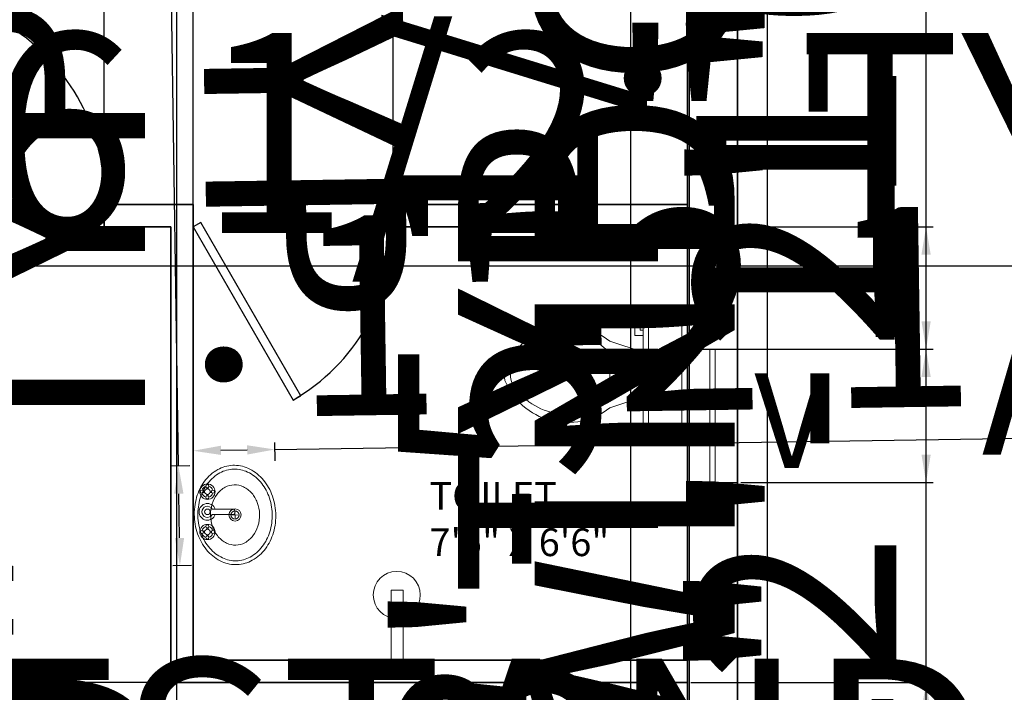
# Model space of a CAD drawing. Units: inches. Extents: x 2901 to 21549, y 2042 to 3828.
# Tile 6 of 10: x 3505 to 3682, y 3226 to 3347. Entities that reach past the tile are written whole.
import ezdxf

# ---------------------------------------------------------------- set-up
doc = ezdxf.new("R2010")
doc.units = ezdxf.units.IN
doc.layers.get('Defpoints').update_dxf_attribs({"color": 1})
for name, color, linetype, lineweight in [('A-ANNO-DIMS', 2, 'Continuous', 18), ('A-ANNO-TEXT', 7, 'Continuous', 18), ('A-AREA-IDEN', 7, 'Continuous', 18), ('A-DOOR', 3, 'Continuous', 25), ('A-FLOR-FIXT', 9, 'Continuous', 18), ('A-GLAZ', 4, 'Continuous', 18), ('A-WALL', 7, 'Continuous', 35)]:
    doc.layers.add(name, color=color, linetype=linetype, lineweight=lineweight)
doc.styles.get("Standard").update_dxf_attribs({"font": 'arial.ttf'})
doc.dimstyles.new('ISO-25', dxfattribs={"dimtxt": 36, "dimasz": 5, "dimexe": 1.25, "dimexo": 0.625, "dimtad": 1, "dimdec": 0, "dimlunit": 3, "dimtxsty": 'Standard', "dimcen": 2.5, "dimadec": 0, "dimazin": 0, "dimtfac": 1, "dimtdec": 0, "dimtmove": 0, "dimatfit": 3, "dimfxl": 1, "dimarcsym": 0})

# ---------------------------------------------------------------- blocks, each defined once
blk = doc.blocks.new('*U21')
for p, q in [((0, 0), (0, -6)), ((40, 0), (40, -6))]:
    blk.add_line(p, q)
blk.add_lwpolyline([(0, 0), (20, 34.64), (21.52, 33.77), (1.52, -0.88)], close=True)
blk.add_arc((0, 0), 40, 0, 60)
blk = doc.blocks.new('*U19')
for p, q in [((0, 0), (0, 6)), ((40, 0), (40, 6))]:
    blk.add_line(p, q)
blk.add_lwpolyline([(0, 0), (20, -34.64), (21.52, -33.77), (1.52, 0.88)], close=True)
blk.add_arc((0, 0), 40, 300, 0)
blk = doc.blocks.new('Toilet - top')
for p, q in [((9.5, -6), (9.5, -2)), ((-10, -8.5), (-8, -8.5)), ((-10, -9.5), (-10, -8.5)), ((-8, -8.5), (-8, -8)), ((-7, -8), (-7, -9.5)), ((-4, -8), (-6, -14)), ((4, -8), (6, -14)), ((-7, -9.5), (-10, -9.5)), ((4, -14), (-4, -14))]:
    blk.add_line(p, q)
blk.add_lwpolyline([(10.5, -8), (10.5, 0), (-10.5, 0), (-10.5, -8)], close=True)
for points in [[(8.5, -1), (-8.5, -1)], [(-9.5, -2), (-9.5, -6)], [(-8.5, -7), (8.5, -7)]]:
    blk.add_lwpolyline(points)
for centre, radius, start, end in [((-8.62, -1.88), 0.884, 81.8699, 188.1301), ((8.62, -1.88), 0.884, 351.8699, 98.1301), ((-8.62, -6.12), 0.884, 171.8699, 278.1301), ((8.62, -6.12), 0.884, 261.8699, 8.1301), ((3.52, -21.58), 12.17, 141.4691, 247.9714), ((4.2, -21.82), 11.33, 136.3677, 238.9468), ((-3.52, -21.58), 12.17, 292.0284, 38.5307), ((-4.2, -21.82), 11.33, 301.053, 43.6321), ((0, -27.88), 4, 245.7318, 294.2682), ((0, -29), 4, 254.8605, 285.1395)]:
    blk.add_arc(centre, radius, start, end)
blk = doc.blocks.new('Sink - Oval top')
for p, q in [((-1, 0), (1, 0)), ((0, 1), (0, -1))]:
    blk.add_line(p, q)
for points in [[(-12.23, 0.39, 0.117634), (-11.46, -3.36, 0.104469), (-8.88, -6.8, 0.090016), (-5.08, -9.07, 0.08192), (-0.32, -10.02, 0.08192), (4.49, -9.38, 0.090016), (8.42, -7.36, 0.104469), (11.22, -4.09, 0.117634), (12.23, -0.39, 0.117634), (11.46, 3.36, 0.104469), (8.88, 6.8, 0.090016), (5.08, 9.07, 0.08192), (0.32, 10.02, 0.08192), (-4.49, 9.38, 0.090016), (-8.42, 7.36, 0.104469), (-11.22, 4.09, 0.117634)], [(-11.29, 0.16, 0.118622), (-10.52, -3.25, 0.104678), (-8.07, -6.36, 0.089562), (-4.54, -8.37, 0.081185), (-0.13, -9.15, 0.081185), (4.3, -8.49, 0.089562), (7.89, -6.58, 0.104678), (10.42, -3.55, 0.118622), (11.29, -0.16, 0.118622), (10.52, 3.25, 0.104678), (8.07, 6.36, 0.089562), (4.54, 8.37, 0.081185), (0.13, 9.15, 0.081185), (-4.3, 8.49, 0.089562), (-7.89, 6.58, 0.104678), (-10.42, 3.55, 0.118622)], [(-7.42, 0.08, 0.118283), (-6.91, -2.17, 0.104607), (-5.29, -4.21, 0.089718), (-2.97, -5.53, 0.081436), (-0.07, -6.04, 0.081436), (2.84, -5.59, 0.089718), (5.2, -4.33, 0.104607), (6.86, -2.32, 0.118283), (7.42, -0.08, 0.118283), (6.91, 2.17, 0.104607), (5.29, 4.21, 0.089718), (2.97, 5.53, 0.081436), (0.07, 6.04, 0.081436), (-2.84, 5.59, 0.089718), (-5.2, 4.33, 0.104607), (-6.86, 2.32, 0.118283)]]:
    blk.add_lwpolyline(points, format="xyb", close=True)
for radius in [1.5, 1]:
    blk.add_circle((0, 0), radius)
blk = doc.blocks.new('Faucet - Bathroom top')
for p, q in [((-4.107, 0.125), (-4.375, 0.125)), ((-3.75, 0.4788), (-3.75, 0.75)), ((-3.5, 0.482), (-3.5, 0.75)), ((-3.1461, 0.125), (-2.875, 0.125)), ((3.143, 0.125), (2.875, 0.125)), ((3.5, 0.4788), (3.5, 0.75)), ((3.75, 0.482), (3.75, 0.75)), ((4.1039, 0.125), (4.375, 0.125)), ((-4.1039, -0.125), (-4.375, -0.125)), ((-3.75, -0.4821), (-3.75, -0.75)), ((-3.5, -0.4789), (-3.5, -0.75)), ((-3.143, -0.125), (-2.875, -0.125)), ((-0.5, -0.8639), (-0.5, -4.5)), ((0.5, -4.5), (0.5, -0.8631)), ((3.1461, -0.125), (2.875, -0.125)), ((3.5, -0.4821), (3.5, -0.75)), ((3.75, -0.4789), (3.75, -0.75)), ((4.107, -0.125), (4.375, -0.125))]:
    blk.add_line(p, q)
for centre, radius in [((-3.625, 0), 1.375), ((-4.625, 0), 0.2795), ((-3.625, 0), 0.5), ((-3.625, 1), 0.2795), ((-2.625, 0), 0.2795), ((0, 0), 0.5), ((3.625, 0), 1.375), ((2.625, 0), 0.2795), ((3.625, 0), 0.5), ((3.625, 1), 0.2795), ((4.625, 0), 0.2795), ((-3.625, -1), 0.2795), ((3.625, -1), 0.2795)]:
    blk.add_circle(centre, radius)
for centre, radius, start, end in [((-3.625, 0), 1, 105.2407, 164.2093), ((-3.625, 0), 1, 16.44125, 74.07887), ((0, 0), 1.5, 289.6514, 250.3603), ((0, 0), 1, 300.3431, 239.7554), ((3.625, 0), 1, 106.12, 164.0884), ((3.625, 0), 1, 16.23422, 73.90469), ((-3.625, 0), 1, 196.2342, 253.9047), ((-3.625, 0), 1, 286.12, 344.0884), ((3.625, 0), 1, 196.4413, 254.0789), ((3.625, 0), 1, 285.2407, 344.2093), ((0, -4.5), 0.5, 180, 0)]:
    blk.add_arc(centre, radius, start, end)
blk = doc.blocks.new('*D36')
at = {"layer": 'A-ANNO-DIMS', "color": 0, "lineweight": -2, "transparency": 16777216}
for p, q in [((3639.47, 3192.64), (3639.47, 3654.44)), ((3634.69, 3192.64), (3640.72, 3192.64)), ((3639.47, 3161.64), (3639.47, 3187.64)), ((3634.69, 3156.64), (3640.72, 3156.64))]:
    blk.add_line(p, q, dxfattribs=at)
at = {"layer": 'A-ANNO-DIMS', "color": 0, "transparency": 16777216}
for points in [[(3638.64, 3187.64), (3640.3, 3187.64), (3639.47, 3192.64)], [(3638.64, 3161.64), (3640.3, 3161.64), (3639.47, 3156.64)]]:
    blk.add_solid(points, dxfattribs=at)
at = {"layer": 'Defpoints', "color": 0, "transparency": 16777216}
for p in [(3634.07, 3192.64), (3639.47, 3192.64), (3634.07, 3156.64)]:
    blk.add_point(p, dxfattribs=at)
at = {"layer": 'A-ANNO-DIMS', "color": 0, "transparency": 16777216, "insert": (3620.21, 3426.04), "char_height": 36, "attachment_point": 5, "rotation": 90}
blk.add_mtext('WINDOW 3\'-0" TYP.', dxfattribs=at)
blk = doc.blocks.new('*D38')
at = {"layer": 'A-ANNO-DIMS', "color": 0, "lineweight": -2, "transparency": 16777216}
for p, q in [((3343.07, 3191.34), (3343.07, 3188.58)), ((3357.29, 3191.34), (3357.29, 3188.58)), ((3348.07, 3189.83), (3352.29, 3189.83)), ((3357.29, 3189.83), (3922.11, 3189.83))]:
    blk.add_line(p, q, dxfattribs=at)
at = {"layer": 'A-ANNO-DIMS', "color": 0, "transparency": 16777216}
for points in [[(3348.07, 3190.67), (3348.07, 3189), (3343.07, 3189.83)], [(3352.29, 3190.67), (3352.29, 3189), (3357.29, 3189.83)]]:
    blk.add_solid(points, dxfattribs=at)
at = {"layer": 'Defpoints', "color": 0, "transparency": 16777216}
for p in [(3343.07, 3191.97), (3357.29, 3191.97), (3357.29, 3189.83)]:
    blk.add_point(p, dxfattribs=at)
at = {"layer": 'A-ANNO-DIMS', "color": 0, "transparency": 16777216, "insert": (3642.2, 3209.07), "char_height": 36, "attachment_point": 5}
blk.add_mtext('NIGHTSTAND 1\'-2" TYP.', dxfattribs=at)
blk = doc.blocks.new('*D42')
at = {"layer": 'A-ANNO-DIMS', "color": 0, "lineweight": -2, "transparency": 16777216}
for p, q in [((3533.42, 3266.44), (3528.38, 3599.53)), ((3535.49, 3266.47), (3532.17, 3266.42)), ((3533.62, 3253.49), (3533.5, 3261.44)), ((3535.76, 3248.52), (3532.44, 3248.47))]:
    blk.add_line(p, q, dxfattribs=at)
at = {"layer": 'A-ANNO-DIMS', "color": 0, "transparency": 16777216}
for points in [[(3534.33, 3261.45), (3532.66, 3261.43), (3533.42, 3266.44)], [(3534.45, 3253.5), (3532.78, 3253.48), (3533.69, 3248.49)]]:
    blk.add_solid(points, dxfattribs=at)
at = {"layer": 'Defpoints', "color": 0, "transparency": 16777216}
for p in [(3533.42, 3266.44), (3536.11, 3266.48), (3536.39, 3248.53)]:
    blk.add_point(p, dxfattribs=at)
at = {"layer": 'A-ANNO-DIMS', "color": 0, "transparency": 16777216, "insert": (3549.86, 3435.77), "char_height": 36, "attachment_point": 5, "rotation": 270.8679}
blk.add_mtext('LAV 1\'-6" TYP.', dxfattribs=at)
blk = doc.blocks.new('*D43')
at = {"layer": 'A-ANNO-DIMS', "color": 0, "lineweight": -2, "transparency": 16777216}
for p, q in [((3550.8, 3269.4), (3856.95, 3274.04)), ((3536.1, 3267.11), (3536.05, 3270.42)), ((3550.83, 3267.33), (3550.78, 3270.65)), ((3541.07, 3269.25), (3545.8, 3269.32))]:
    blk.add_line(p, q, dxfattribs=at)
at = {"layer": 'A-ANNO-DIMS', "color": 0, "transparency": 16777216}
for points in [[(3541.06, 3270.08), (3541.09, 3268.42), (3536.07, 3269.17)], [(3545.78, 3270.16), (3545.81, 3268.49), (3550.8, 3269.4)]]:
    blk.add_solid(points, dxfattribs=at)
at = {"layer": 'Defpoints', "color": 0, "transparency": 16777216}
for p in [(3550.8, 3269.4), (3536.11, 3266.48), (3550.84, 3266.71)]:
    blk.add_point(p, dxfattribs=at)
at = {"layer": 'A-ANNO-DIMS', "color": 0, "transparency": 16777216, "insert": (3706.08, 3290.99), "char_height": 36, "attachment_point": 5, "rotation": 0.8679}
blk.add_mtext('1\'-2 1/2" TYP.', dxfattribs=at)
blk = doc.blocks.new('*D45')
at = {"layer": 'A-ANNO-DIMS', "color": 0, "lineweight": -2, "transparency": 16777216}
for p, q in [((3419.19, 3302.47), (3414.19, 3302.47)), ((3424.19, 3301.6), (3424.19, 3303.72)), ((3424.19, 3302.47), (3430.69, 3302.47)), ((3430.69, 3301.6), (3430.69, 3303.72)), ((3435.69, 3302.47), (3745.26, 3302.47))]:
    blk.add_line(p, q, dxfattribs=at)
at = {"layer": 'A-ANNO-DIMS', "color": 0, "transparency": 16777216}
for points in [[(3419.19, 3303.31), (3419.19, 3301.64), (3424.19, 3302.47)], [(3435.69, 3303.31), (3435.69, 3301.64), (3430.69, 3302.47)]]:
    blk.add_solid(points, dxfattribs=at)
at = {"layer": 'Defpoints', "color": 0, "transparency": 16777216}
for p in [(3430.69, 3302.47), (3424.19, 3300.97), (3430.69, 3300.97)]:
    blk.add_point(p, dxfattribs=at)
at = {"layer": 'A-ANNO-DIMS', "color": 0, "transparency": 16777216, "insert": (3592.98, 3321.71), "char_height": 36, "attachment_point": 5}
blk.add_mtext('0\'-6 1/2" TYP.', dxfattribs=at)
blk = doc.blocks.new('*D46')
at = {"layer": 'A-ANNO-DIMS', "color": 0, "lineweight": -2, "transparency": 16777216}
for p, q in [((3545.07, 3370.05), (3545.07, 3357.42)), ((3625.07, 3370.05), (3625.07, 3357.42)), ((3550.07, 3358.67), (3620.07, 3358.67)), ((3625.07, 3358.67), (4160.88, 3358.67))]:
    blk.add_line(p, q, dxfattribs=at)
at = {"layer": 'A-ANNO-DIMS', "color": 0, "transparency": 16777216}
for points in [[(3550.07, 3359.51), (3550.07, 3357.84), (3545.07, 3358.67)], [(3620.07, 3359.51), (3620.07, 3357.84), (3625.07, 3358.67)]]:
    blk.add_solid(points, dxfattribs=at)
at = {"layer": 'Defpoints', "color": 0, "transparency": 16777216}
for p in [(3545.07, 3370.67), (3625.07, 3370.67), (3625.07, 3358.67)]:
    blk.add_point(p, dxfattribs=at)
at = {"layer": 'A-ANNO-DIMS', "color": 0, "transparency": 16777216, "insert": (3895.48, 3379.02), "char_height": 36, "attachment_point": 5}
blk.add_mtext('QUEEN BED 6\'-8" TYP.', dxfattribs=at)
blk = doc.blocks.new('*D47')
at = {"layer": 'A-ANNO-DIMS', "color": 0, "lineweight": -2, "transparency": 16777216}
for p, q in [((3544.44, 3430.67), (3531.82, 3430.67)), ((3533.07, 3425.67), (3533.07, 3375.67)), ((3544.44, 3370.67), (3531.82, 3370.67)), ((3533.07, 3370.67), (3533.07, 3144.99))]:
    blk.add_line(p, q, dxfattribs=at)
at = {"layer": 'A-ANNO-DIMS', "color": 0, "transparency": 16777216}
for points in [[(3532.24, 3425.67), (3533.9, 3425.67), (3533.07, 3430.67)], [(3532.24, 3375.67), (3533.9, 3375.67), (3533.07, 3370.67)]]:
    blk.add_solid(points, dxfattribs=at)
at = {"layer": 'Defpoints', "color": 0, "transparency": 16777216}
for p in [(3545.07, 3430.67), (3533.07, 3370.67), (3545.07, 3370.67)]:
    blk.add_point(p, dxfattribs=at)
at = {"layer": 'A-ANNO-DIMS', "color": 0, "transparency": 16777216, "insert": (3514.06, 3255.33), "char_height": 36, "attachment_point": 5, "rotation": 90}
blk.add_mtext('5\'-0" TYP.', dxfattribs=at)
blk = doc.blocks.new('*D50')
at = {"layer": 'A-ANNO-DIMS', "color": 0, "lineweight": -2, "transparency": 16777216}
for p, q in [((3599.61, 3100.68), (3599.61, 3096.69)), ((3622.08, 3100.68), (3622.08, 3096.69)), ((3604.61, 3097.94), (3617.08, 3097.94)), ((3622.08, 3097.94), (4251.18, 3097.94))]:
    blk.add_line(p, q, dxfattribs=at)
at = {"layer": 'A-ANNO-DIMS', "color": 0, "transparency": 16777216}
for points in [[(3604.61, 3098.77), (3604.61, 3097.1), (3599.61, 3097.94)], [(3617.08, 3098.77), (3617.08, 3097.1), (3622.08, 3097.94)]]:
    blk.add_solid(points, dxfattribs=at)
at = {"layer": 'Defpoints', "color": 0, "transparency": 16777216}
for p in [(3599.61, 3101.31), (3622.08, 3101.31), (3622.08, 3097.94)]:
    blk.add_point(p, dxfattribs=at)
at = {"layer": 'A-ANNO-DIMS', "color": 0, "transparency": 16777216, "insert": (3939.13, 3117.18), "char_height": 36, "attachment_point": 5}
blk.add_mtext('END TABLE 1\'-10 1/2" TYP.', dxfattribs=at)
blk = doc.blocks.new('*D51')
at = {"layer": 'A-ANNO-DIMS', "color": 0, "lineweight": -2, "transparency": 16777216}
for p, q in [((3625.45, 3119.55), (3625.45, 3341.85)), ((3622.7, 3119.55), (3626.7, 3119.55)), ((3625.45, 3106.31), (3625.45, 3114.55)), ((3622.7, 3101.31), (3626.7, 3101.31))]:
    blk.add_line(p, q, dxfattribs=at)
at = {"layer": 'A-ANNO-DIMS', "color": 0, "transparency": 16777216}
for points in [[(3624.61, 3114.55), (3626.28, 3114.55), (3625.45, 3119.55)], [(3624.61, 3106.31), (3626.28, 3106.31), (3625.45, 3101.31)]]:
    blk.add_solid(points, dxfattribs=at)
at = {"layer": 'Defpoints', "color": 0, "transparency": 16777216}
for p in [(3622.08, 3119.55), (3625.45, 3119.55), (3622.08, 3101.31)]:
    blk.add_point(p, dxfattribs=at)
at = {"layer": 'A-ANNO-DIMS', "color": 0, "transparency": 16777216, "insert": (3606.44, 3233.2), "char_height": 36, "attachment_point": 5, "rotation": 90}
blk.add_mtext('1\'-6" TYP.', dxfattribs=at)
blk = doc.blocks.new('*D54')
at = {"layer": 'A-ANNO-DIMS', "color": 0, "lineweight": -2, "transparency": 16777216}
for p, q in [((3536.12, 3164.87), (3536.12, 3153.97)), ((3604.61, 3164.87), (3604.61, 3153.97)), ((3541.12, 3155.22), (3599.61, 3155.22)), ((3604.61, 3155.22), (4090.43, 3155.22))]:
    blk.add_line(p, q, dxfattribs=at)
at = {"layer": 'A-ANNO-DIMS', "color": 0, "transparency": 16777216}
for points in [[(3541.12, 3156.05), (3541.12, 3154.38), (3536.12, 3155.22)], [(3599.61, 3156.05), (3599.61, 3154.38), (3604.61, 3155.22)]]:
    blk.add_solid(points, dxfattribs=at)
at = {"layer": 'Defpoints', "color": 0, "transparency": 16777216}
for p in [(3536.12, 3165.49), (3604.61, 3165.49), (3604.61, 3155.22)]:
    blk.add_point(p, dxfattribs=at)
at = {"layer": 'A-ANNO-DIMS', "color": 0, "transparency": 16777216, "insert": (3850.02, 3174.46), "char_height": 36, "attachment_point": 5}
blk.add_mtext('DINING SET 5\'-8 1/2"', dxfattribs=at)
blk = doc.blocks.new('*D55')
at = {"layer": 'A-ANNO-DIMS', "color": 0, "lineweight": -2, "transparency": 16777216}
for p, q in [((3614.88, 3206.89), (3614.88, 3392.69)), ((3605.24, 3206.89), (3616.13, 3206.89)), ((3614.88, 3170.49), (3614.88, 3201.89)), ((3605.24, 3165.49), (3616.13, 3165.49))]:
    blk.add_line(p, q, dxfattribs=at)
at = {"layer": 'A-ANNO-DIMS', "color": 0, "transparency": 16777216}
for points in [[(3614.05, 3201.89), (3615.72, 3201.89), (3614.88, 3206.89)], [(3614.05, 3170.49), (3615.72, 3170.49), (3614.88, 3165.49)]]:
    blk.add_solid(points, dxfattribs=at)
at = {"layer": 'Defpoints', "color": 0, "transparency": 16777216}
for p in [(3604.61, 3206.89), (3614.88, 3206.89), (3604.61, 3165.49)]:
    blk.add_point(p, dxfattribs=at)
at = {"layer": 'A-ANNO-DIMS', "color": 0, "transparency": 16777216, "insert": (3595.63, 3302.29), "char_height": 36, "attachment_point": 5, "rotation": 90}
blk.add_mtext('3\'-5 1/2"', dxfattribs=at)
blk = doc.blocks.new('*D67')
at = {"layer": 'A-ANNO-DIMS', "color": 0, "lineweight": -2, "transparency": 16777216}
for p, q in [((3484.07, 3013.1), (3484.07, 3509.68)), ((3489.07, 3508.43), (3620.07, 3508.43)), ((3625.07, 3228.1), (3625.07, 3509.68))]:
    blk.add_line(p, q, dxfattribs=at)
at = {"layer": 'A-ANNO-DIMS', "color": 0, "transparency": 16777216}
for points in [[(3489.07, 3509.26), (3489.07, 3507.59), (3484.07, 3508.43)], [(3620.07, 3509.26), (3620.07, 3507.59), (3625.07, 3508.43)]]:
    blk.add_solid(points, dxfattribs=at)
at = {"layer": 'Defpoints', "color": 0, "transparency": 16777216}
for p in [(3625.07, 3508.43), (3625.07, 3227.48), (3484.07, 3012.48)]:
    blk.add_point(p, dxfattribs=at)
at = {"layer": 'A-ANNO-DIMS', "color": 0, "transparency": 16777216, "insert": (3554.57, 3527.43), "char_height": 36, "attachment_point": 5}
blk.add_mtext('11\'-9"', dxfattribs=at)
blk = doc.blocks.new('*D68')
at = {"layer": 'A-ANNO-DIMS', "color": 0, "lineweight": -2, "transparency": 16777216}
for p, q in [((3531.44, 3227.48), (3298.87, 3227.48)), ((3300.12, 3017.48), (3300.12, 3222.48)), ((3483.44, 3012.48), (3298.87, 3012.48))]:
    blk.add_line(p, q, dxfattribs=at)
at = {"layer": 'A-ANNO-DIMS', "color": 0, "transparency": 16777216}
for points in [[(3299.29, 3222.48), (3300.95, 3222.48), (3300.12, 3227.48)], [(3299.29, 3017.48), (3300.95, 3017.48), (3300.12, 3012.48)]]:
    blk.add_solid(points, dxfattribs=at)
at = {"layer": 'Defpoints', "color": 0, "transparency": 16777216}
for p in [(3300.12, 3227.48), (3532.07, 3227.48), (3484.07, 3012.48)]:
    blk.add_point(p, dxfattribs=at)
at = {"layer": 'A-ANNO-DIMS', "color": 0, "transparency": 16777216, "insert": (3281.42, 3119.98), "char_height": 36, "attachment_point": 5, "rotation": 90}
blk.add_mtext('17\'-11"', dxfattribs=at)
blk = doc.blocks.new('*D69')
at = {"layer": 'A-ANNO-DIMS', "color": 0, "lineweight": -2, "transparency": 16777216}
for p, q in [((3668.02, 3287.47), (3668.02, 3390.03)), ((3634.69, 3287.47), (3669.27, 3287.47)), ((3668.02, 3268.47), (3668.02, 3282.47)), ((3634.69, 3263.47), (3669.27, 3263.47))]:
    blk.add_line(p, q, dxfattribs=at)
at = {"layer": 'A-ANNO-DIMS', "color": 0, "transparency": 16777216}
for points in [[(3667.19, 3282.47), (3668.85, 3282.47), (3668.02, 3287.47)], [(3667.19, 3268.47), (3668.85, 3268.47), (3668.02, 3263.47)]]:
    blk.add_solid(points, dxfattribs=at)
at = {"layer": 'Defpoints', "color": 0, "transparency": 16777216}
for p in [(3634.07, 3287.47), (3668.02, 3287.47), (3634.07, 3263.47)]:
    blk.add_point(p, dxfattribs=at)
at = {"layer": 'A-ANNO-DIMS', "color": 0, "transparency": 16777216, "insert": (3649.01, 3341.25), "char_height": 36, "attachment_point": 5, "rotation": 90}
blk.add_mtext('2\'-0"', dxfattribs=at)
blk = doc.blocks.new('*D70')
at = {"layer": 'A-ANNO-DIMS', "color": 0, "lineweight": -2, "transparency": 16777216}
for p, q in [((3668.02, 3309.48), (3668.02, 3436.01)), ((3625.69, 3309.48), (3669.27, 3309.48)), ((3668.02, 3292.47), (3668.02, 3304.48)), ((3625.69, 3287.47), (3669.27, 3287.47))]:
    blk.add_line(p, q, dxfattribs=at)
at = {"layer": 'A-ANNO-DIMS', "color": 0, "transparency": 16777216}
for points in [[(3667.19, 3304.48), (3668.85, 3304.48), (3668.02, 3309.48)], [(3667.19, 3292.47), (3668.85, 3292.47), (3668.02, 3287.47)]]:
    blk.add_solid(points, dxfattribs=at)
at = {"layer": 'Defpoints', "color": 0, "transparency": 16777216}
for p in [(3625.07, 3309.48), (3668.02, 3309.48), (3625.07, 3287.47)]:
    blk.add_point(p, dxfattribs=at)
at = {"layer": 'A-ANNO-DIMS', "color": 0, "transparency": 16777216, "insert": (3649.01, 3375.24), "char_height": 36, "attachment_point": 5, "rotation": 90}
blk.add_mtext('1\'-10"', dxfattribs=at)
blk = doc.blocks.new('*D71')
at = {"layer": 'A-ANNO-DIMS', "color": 0, "lineweight": -2, "transparency": 16777216}
for p, q in [((3536.07, 3310.1), (3536.07, 3509.68)), ((3541.07, 3508.43), (3567.07, 3508.43)), ((3572.07, 3310.1), (3572.07, 3509.68)), ((3572.07, 3508.43), (3673.99, 3508.43))]:
    blk.add_line(p, q, dxfattribs=at)
at = {"layer": 'A-ANNO-DIMS', "color": 0, "transparency": 16777216}
for points in [[(3541.07, 3509.26), (3541.07, 3507.59), (3536.07, 3508.43)], [(3567.07, 3509.26), (3567.07, 3507.59), (3572.07, 3508.43)]]:
    blk.add_solid(points, dxfattribs=at)
at = {"layer": 'Defpoints', "color": 0, "transparency": 16777216}
for p in [(3572.07, 3508.43), (3536.07, 3309.48), (3572.07, 3309.48)]:
    blk.add_point(p, dxfattribs=at)
at = {"layer": 'A-ANNO-DIMS', "color": 0, "transparency": 16777216, "insert": (3625.53, 3527.45), "char_height": 36, "attachment_point": 5}
blk.add_mtext('3\'-0"', dxfattribs=at)
blk = doc.blocks.new('*D73')
at = {"layer": 'A-ANNO-DIMS', "color": 0, "lineweight": -2, "transparency": 16777216}
for p, q in [((3668.02, 3058.19), (3668.02, 3244)), ((3625.69, 3058.19), (3669.27, 3058.19)), ((3668.02, 3017.48), (3668.02, 3053.19)), ((3625.69, 3012.48), (3669.27, 3012.48))]:
    blk.add_line(p, q, dxfattribs=at)
at = {"layer": 'A-ANNO-DIMS', "color": 0, "transparency": 16777216}
for points in [[(3667.19, 3053.19), (3668.85, 3053.19), (3668.02, 3058.19)], [(3667.19, 3017.48), (3668.85, 3017.48), (3668.02, 3012.48)]]:
    blk.add_solid(points, dxfattribs=at)
at = {"layer": 'Defpoints', "color": 0, "transparency": 16777216}
for p in [(3625.07, 3058.19), (3668.02, 3058.19), (3625.07, 3012.48)]:
    blk.add_point(p, dxfattribs=at)
at = {"layer": 'A-ANNO-DIMS', "color": 0, "transparency": 16777216, "insert": (3648.77, 3153.6), "char_height": 36, "attachment_point": 5, "rotation": 90}
blk.add_mtext('3\'-9 1/2"', dxfattribs=at)
blk = doc.blocks.new('*D74')
at = {"layer": 'A-ANNO-DIMS', "color": 0, "lineweight": -2, "transparency": 16777216}
for p, q in [((3668.02, 3227.48), (3668.02, 3358.01)), ((3625.69, 3227.48), (3669.27, 3227.48)), ((3668.02, 3197.64), (3668.02, 3222.48)), ((3625.69, 3192.64), (3669.27, 3192.64))]:
    blk.add_line(p, q, dxfattribs=at)
at = {"layer": 'A-ANNO-DIMS', "color": 0, "transparency": 16777216}
for points in [[(3667.19, 3222.48), (3668.85, 3222.48), (3668.02, 3227.48)], [(3667.19, 3197.64), (3668.85, 3197.64), (3668.02, 3192.64)]]:
    blk.add_solid(points, dxfattribs=at)
at = {"layer": 'Defpoints', "color": 0, "transparency": 16777216}
for p in [(3625.07, 3227.48), (3668.02, 3227.48), (3625.07, 3192.64)]:
    blk.add_point(p, dxfattribs=at)
at = {"layer": 'A-ANNO-DIMS', "color": 0, "transparency": 16777216, "insert": (3649.32, 3295.24), "char_height": 36, "attachment_point": 5, "rotation": 90}
blk.add_mtext('2\'-11"', dxfattribs=at)
blk = doc.blocks.new('*D77')
at = {"layer": 'A-ANNO-DIMS', "color": 0, "lineweight": -2, "transparency": 16777216}
for p, q in [((3475.07, 3508.43), (3470.07, 3508.43)), ((3480.07, 3310.1), (3480.07, 3509.68)), ((3480.07, 3508.43), (3484.07, 3508.43)), ((3484.07, 3310.1), (3484.07, 3509.68)), ((3489.07, 3508.43), (3591.02, 3508.43))]:
    blk.add_line(p, q, dxfattribs=at)
at = {"layer": 'A-ANNO-DIMS', "color": 0, "transparency": 16777216}
for points in [[(3475.07, 3509.26), (3475.07, 3507.59), (3480.07, 3508.43)], [(3489.07, 3509.26), (3489.07, 3507.59), (3484.07, 3508.43)]]:
    blk.add_solid(points, dxfattribs=at)
at = {"layer": 'Defpoints', "color": 0, "transparency": 16777216}
for p in [(3484.07, 3508.43), (3480.07, 3309.48), (3484.07, 3309.48)]:
    blk.add_point(p, dxfattribs=at)
at = {"layer": 'A-ANNO-DIMS', "color": 0, "transparency": 16777216, "insert": (3542.54, 3527.43), "char_height": 36, "attachment_point": 5}
blk.add_mtext('0\'-4"', dxfattribs=at)
blk = doc.blocks.new('*D78')
at = {"layer": 'A-ANNO-DIMS', "color": 0, "lineweight": -2, "transparency": 16777216}
for p, q in [((3343.07, 3230.85), (3343.07, 2839.28)), ((3366.66, 3230.85), (3366.66, 2839.28)), ((3348.07, 2840.53), (3361.66, 2840.53)), ((3366.66, 2840.53), (3577.07, 2840.53))]:
    blk.add_line(p, q, dxfattribs=at)
at = {"layer": 'A-ANNO-DIMS', "color": 0, "transparency": 16777216}
for points in [[(3348.07, 2841.36), (3348.07, 2839.69), (3343.07, 2840.53)], [(3361.66, 2841.36), (3361.66, 2839.69), (3366.66, 2840.53)]]:
    blk.add_solid(points, dxfattribs=at)
at = {"layer": 'Defpoints', "color": 0, "transparency": 16777216}
for p in [(3343.07, 3231.48), (3366.66, 3231.48), (3366.66, 2840.53)]:
    blk.add_point(p, dxfattribs=at)
at = {"layer": 'A-ANNO-DIMS', "color": 0, "transparency": 16777216, "insert": (3474.37, 2859.77), "char_height": 36, "attachment_point": 5}
blk.add_mtext('1\'-11 1/2"', dxfattribs=at)
blk = doc.blocks.new('*D81')
at = {"layer": 'A-ANNO-DIMS', "color": 0, "lineweight": -2, "transparency": 16777216}
for p, q in [((3444.07, 3314.1), (3444.07, 3509.68)), ((3449.07, 3508.43), (3475.07, 3508.43)), ((3480.07, 3314.1), (3480.07, 3509.68)), ((3480.07, 3508.43), (3581.99, 3508.43))]:
    blk.add_line(p, q, dxfattribs=at)
at = {"layer": 'A-ANNO-DIMS', "color": 0, "transparency": 16777216}
for points in [[(3449.07, 3509.26), (3449.07, 3507.59), (3444.07, 3508.43)], [(3475.07, 3509.26), (3475.07, 3507.59), (3480.07, 3508.43)]]:
    blk.add_solid(points, dxfattribs=at)
at = {"layer": 'Defpoints', "color": 0, "transparency": 16777216}
for p in [(3480.07, 3508.43), (3444.07, 3313.48), (3480.07, 3313.48)]:
    blk.add_point(p, dxfattribs=at)
at = {"layer": 'A-ANNO-DIMS', "color": 0, "transparency": 16777216, "insert": (3533.53, 3527.45), "char_height": 36, "attachment_point": 5}
blk.add_mtext('3\'-0"', dxfattribs=at)
blk = doc.blocks.new('*D82')
at = {"layer": 'A-ANNO-DIMS', "color": 0, "lineweight": -2, "transparency": 16777216}
for p, q in [((3484.07, 3313.93), (3484.07, 3509.68)), ((3489.07, 3508.43), (3515.07, 3508.43)), ((3520.07, 3314.1), (3520.07, 3509.68)), ((3520.07, 3508.43), (3621.99, 3508.43))]:
    blk.add_line(p, q, dxfattribs=at)
at = {"layer": 'A-ANNO-DIMS', "color": 0, "transparency": 16777216}
for points in [[(3489.07, 3509.26), (3489.07, 3507.59), (3484.07, 3508.43)], [(3515.07, 3509.26), (3515.07, 3507.59), (3520.07, 3508.43)]]:
    blk.add_solid(points, dxfattribs=at)
at = {"layer": 'Defpoints', "color": 0, "transparency": 16777216}
for p in [(3520.07, 3508.43), (3484.07, 3313.3), (3520.07, 3313.48)]:
    blk.add_point(p, dxfattribs=at)
at = {"layer": 'A-ANNO-DIMS', "color": 0, "transparency": 16777216, "insert": (3573.53, 3527.45), "char_height": 36, "attachment_point": 5}
blk.add_mtext('3\'-0"', dxfattribs=at)
blk = doc.blocks.new('*D84')
at = {"layer": 'A-ANNO-DIMS', "color": 0, "lineweight": -2, "transparency": 16777216}
for p, q in [((3444.07, 3230.85), (3444.07, 2839.28)), ((3480.07, 3230.85), (3480.07, 2839.28)), ((3449.07, 2840.53), (3475.07, 2840.53)), ((3480.07, 2840.53), (3581.99, 2840.53))]:
    blk.add_line(p, q, dxfattribs=at)
at = {"layer": 'A-ANNO-DIMS', "color": 0, "transparency": 16777216}
for points in [[(3449.07, 2841.36), (3449.07, 2839.69), (3444.07, 2840.53)], [(3475.07, 2841.36), (3475.07, 2839.69), (3480.07, 2840.53)]]:
    blk.add_solid(points, dxfattribs=at)
at = {"layer": 'Defpoints', "color": 0, "transparency": 16777216}
for p in [(3444.07, 3231.48), (3480.07, 3231.48), (3480.07, 2840.53)]:
    blk.add_point(p, dxfattribs=at)
at = {"layer": 'A-ANNO-DIMS', "color": 0, "transparency": 16777216, "insert": (3533.53, 2859.55), "char_height": 36, "attachment_point": 5}
blk.add_mtext('3\'-0"', dxfattribs=at)

msp = doc.modelspace()

# ---------------------------------------------------------------- linework, layer by layer
at = {"layer": 'A-FLOR-FIXT'}
for p, q in [((3573.9, 3244.1), (3571.73, 3244.1)), ((3571.73, 3244.1), (3571.73, 3231.48)), ((3573.9, 3231.48), (3573.9, 3244.1))]:
    msp.add_line(p, q, dxfattribs=at)
msp.add_circle((3572.72, 3243.23), 4.23, dxfattribs=at)
at = {"layer": 'A-GLAZ'}
for p, q in [((3625.07, 3287.47), (3634.07, 3287.47)), ((3625.07, 3263.47), (3625.07, 3287.47)), ((3629.07, 3263.47), (3629.07, 3287.47)), ((3630.07, 3287.47), (3630.07, 3263.47)), ((3634.07, 3287.47), (3634.07, 3263.47)), ((3634.07, 3263.47), (3625.07, 3263.47))]:
    msp.add_line(p, q, dxfattribs=at)
at = {"layer": 'A-WALL'}
for p, q in [((3625.07, 3465.48), (3625.07, 2883.48)), ((3520.07, 3309.48), (3520.07, 3313.48)), ((3520.07, 3313.48), (3536.07, 3313.48)), ((3536.07, 3309.48), (3536.07, 3313.48)), ((3572.07, 3309.48), (3572.07, 3313.48)), ((3572.07, 3313.48), (3625.07, 3313.48)), ((3520.07, 3309.48), (3532.07, 3309.48)), ((3532.07, 3309.48), (3532.07, 3227.48)), ((3536.07, 3309.48), (3536.07, 3231.48)), ((3536.07, 3309.48), (3536.07, 3231.48)), ((3572.07, 3309.48), (3625.07, 3309.48)), ((3536.07, 3231.48), (3625.07, 3231.48)), ((3532.07, 3227.48), (3625.07, 3227.48))]:
    msp.add_line(p, q, dxfattribs=at)
msp.add_lwpolyline([(3634.07, 3474.48), (3634.07, 2874.48), (3334.07, 2874.48), (3334.07, 3474.48)], close=True, dxfattribs=at)

# ---------------------------------------------------------------- block references
at = {"layer": 'A-DOOR'}
for name, p, xscale, yscale, zscale in [('*U21', (3484.07, 3314.88), 0.8999999999999834, 0.8999999999999834, 0.8999999999999834), ('*U19', (3536.07, 3309.48), 0.9, 0.9, 0.9)]:
    msp.add_blockref(name, p, dxfattribs=dict(at, xscale=xscale, yscale=yscale, zscale=zscale))
at = {"layer": 'A-FLOR-FIXT', "rotation": 270}
msp.add_blockref('Toilet - top', (3625.07, 3282.89), dxfattribs=at)
at = {"layer": 'A-FLOR-FIXT', "xscale": -0.7312020304199782, "yscale": 0.7312020304199782, "zscale": 0.7312020304199782, "rotation": 270.8679213487539}
msp.add_blockref('Sink - Oval top', (3543.61, 3257.62), dxfattribs=at)
at = {"layer": 'A-FLOR-FIXT', "xscale": -1, "rotation": 90}
msp.add_blockref('Faucet - Bathroom top', (3538.64, 3258.18), dxfattribs=at)

# ---------------------------------------------------------------- texts
at = {"layer": 'A-ANNO-TEXT', "insert": (3637.12, 3283.08), "char_height": 17, "attachment_point": 1}
msp.add_mtext_dynamic_manual_height_columns('{\\fArial|b1|i0|c0|p34;V}', width=86.7973, gutter_width=12.5, heights=[27.4], dxfattribs=at)
at = {"layer": 'A-AREA-IDEN', "insert": (3578.62, 3263.55), "char_height": 5, "attachment_point": 1}
msp.add_mtext_dynamic_manual_height_columns('{\\fArial|b1|i0|c0|p34;TOILET\\P7\'5" X 6\'6"}', width=86.7973, gutter_width=12.5, heights=[27.4], dxfattribs=at)

# ---------------------------------------------------------------- dimensions: what is measured, and where the dimension line sits
at = {"layer": 'A-ANNO-DIMS'}
for base, p1, p2, angle, text, picture, middle in [((3639.47, 3192.64), (3634.07, 3156.64), (3634.07, 3192.64), 90, 'WINDOW <> TYP.', '*D36', (3620.21, 3426.04)), ((3533.42, 3266.44), (3536.39, 3248.53), (3536.11, 3266.48), 90.8679, 'LAV <> TYP.', '*D42', (3549.86, 3435.77)), ((3533.07, 3370.67), (3545.07, 3430.67), (3545.07, 3370.67), 270, '<> TYP.', '*D47', (3514.06, 3255.33)), ((3550.8, 3269.4), (3536.11, 3266.48), (3550.84, 3266.71), 0.8679, '<> TYP.', '*D43', (3706.08, 3290.99)), ((3625.45, 3119.55), (3622.08, 3101.31), (3622.08, 3119.55), 90, '<> TYP.', '*D51', (3606.44, 3233.2))]:
    dim = msp.add_linear_dim(base=base, p1=p1, p2=p2, angle=angle, text=text, dimstyle='ISO-25', override={"dimdec": 1, "dimlfac": 1, "dimrnd": 0, "dimzin": 1, "dimdsep": 46, "dimlunit": 4, "dimfrac": 2}, dxfattribs=at)
    dim.commit()
    dim.dimension.update_dxf_attribs({"geometry": picture, "text_midpoint": middle})
for base, p1, p2, picture, middle in [((3480.07, 3508.43), (3444.07, 3313.48), (3480.07, 3313.48), '*D81', (3533.53, 3527.45)), ((3484.07, 3508.43), (3480.07, 3309.48), (3484.07, 3309.48), '*D77', (3542.54, 3527.43)), ((3520.07, 3508.43), (3484.07, 3313.3), (3520.07, 3313.48), '*D82', (3573.53, 3527.45)), ((3625.07, 3508.43), (3484.07, 3012.48), (3625.07, 3227.48), '*D67', (3554.57, 3527.43)), ((3572.07, 3508.43), (3536.07, 3309.48), (3572.07, 3309.48), '*D71', (3625.53, 3527.45)), ((3366.66, 2840.53), (3343.07, 3231.48), (3366.66, 3231.48), '*D78', (3474.37, 2859.77)), ((3480.07, 2840.53), (3444.07, 3231.48), (3480.07, 3231.48), '*D84', (3533.53, 2859.55))]:
    dim = msp.add_linear_dim(base=base, p1=p1, p2=p2, dimstyle='ISO-25', override={"dimdec": 1, "dimlfac": 1, "dimrnd": 0, "dimzin": 1, "dimdsep": 46, "dimlunit": 4, "dimfrac": 2}, dxfattribs=at)
    dim.commit()
    dim.dimension.update_dxf_attribs({"geometry": picture, "text_midpoint": middle})
for base, p1, p2, text, picture, middle in [((3625.07, 3358.67), (3545.07, 3370.67), (3625.07, 3370.67), 'QUEEN BED <> TYP.', '*D46', (3895.48, 3379.02)), ((3430.69, 3302.47), (3424.19, 3300.97), (3430.69, 3300.97), '<> TYP.', '*D45', (3592.98, 3321.71)), ((3357.29, 3189.83), (3343.07, 3191.97), (3357.29, 3191.97), 'NIGHTSTAND <> TYP.', '*D38', (3642.2, 3209.07)), ((3604.61, 3155.22), (3536.12, 3165.49), (3604.61, 3165.49), 'DINING SET <>', '*D54', (3850.02, 3174.46)), ((3622.08, 3097.94), (3599.61, 3101.31), (3622.08, 3101.31), 'END TABLE <> TYP.', '*D50', (3939.13, 3117.18))]:
    dim = msp.add_linear_dim(base=base, p1=p1, p2=p2, text=text, dimstyle='ISO-25', override={"dimdec": 1, "dimlfac": 1, "dimrnd": 0, "dimzin": 1, "dimdsep": 46, "dimlunit": 4, "dimfrac": 2}, dxfattribs=at)
    dim.commit()
    dim.dimension.update_dxf_attribs({"geometry": picture, "text_midpoint": middle})
for base, p1, p2, picture, middle in [((3668.02, 3309.48), (3625.07, 3287.47), (3625.07, 3309.48), '*D70', (3649.01, 3375.24)), ((3668.02, 3287.47), (3634.07, 3263.47), (3634.07, 3287.47), '*D69', (3649.01, 3341.25)), ((3614.88, 3206.89), (3604.61, 3165.49), (3604.61, 3206.89), '*D55', (3595.63, 3302.29)), ((3668.02, 3227.48), (3625.07, 3192.64), (3625.07, 3227.48), '*D74', (3649.32, 3295.24)), ((3668.02, 3058.19), (3625.07, 3012.48), (3625.07, 3058.19), '*D73', (3648.77, 3153.6)), ((3300.12, 3227.48), (3484.07, 3012.48), (3532.07, 3227.48), '*D68', (3281.42, 3119.98))]:
    dim = msp.add_linear_dim(base=base, p1=p1, p2=p2, angle=90, dimstyle='ISO-25', override={"dimdec": 1, "dimlfac": 1, "dimrnd": 0, "dimzin": 1, "dimdsep": 46, "dimlunit": 4, "dimfrac": 2}, dxfattribs=at)
    dim.commit()
    dim.dimension.update_dxf_attribs({"geometry": picture, "text_midpoint": middle})

doc.saveas('drawing.dxf')
